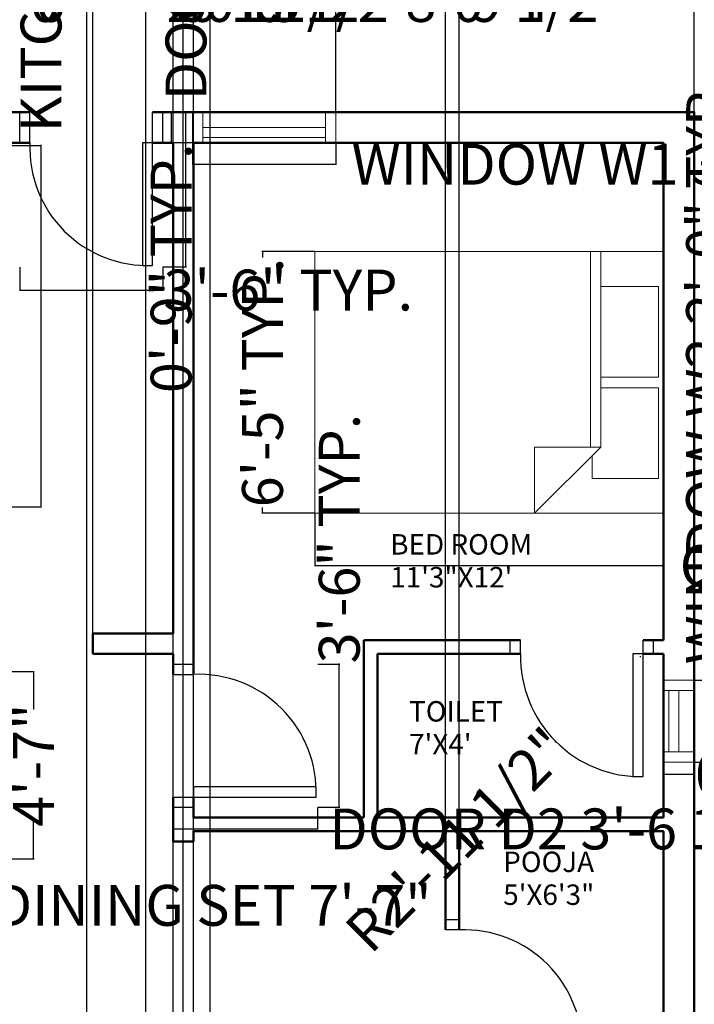
# Model space of a CAD drawing. Units: inches. Extents: x -51 to 1118, y -44 to 791.
# Tile 5 of 8: x 142 to 340, y 344 to 633. Entities that reach past the tile are written whole.
import ezdxf

# ---------------------------------------------------------------- set-up
doc = ezdxf.new("R2010")
doc.units = ezdxf.units.IN
doc.header["$MEASUREMENT"] = 0
for name, color, linetype, lineweight in [('A-ANNO-DIMS', 2, 'Continuous', 18), ('A-AREA-IDEN', 7, 'Continuous', 18), ('A-DOOR', 3, 'Continuous', 25), ('A-FURN', 8, 'Continuous', 18), ('A-GLAZ', 4, 'Continuous', 18), ('A-WALL', 7, 'Continuous', 50)]:
    doc.layers.add(name, color=color, linetype=linetype, lineweight=lineweight)
doc.styles.get("Standard").update_dxf_attribs({"font": 'arial.ttf'})
doc.dimstyles.get("Standard").update_dxf_attribs({"dimtxt": 12, "dimasz": 0.18, "dimexe": 0.18, "dimexo": 0.0625, "dimgap": 0.09, "dimtad": 0, "dimdec": 1, "dimzin": 0, "dimdsep": 46, "dimlunit": 3, "dimtxsty": 'Standard', "dimcen": 0.09, "dimadec": 0, "dimazin": 0, "dimtfac": 1, "dimtdec": 1, "dimtofl": 0, "dimtmove": 0, "dimatfit": 3, "dimfxl": 1, "dimtolj": 1, "dimtzin": 0, "dimarcsym": 0})

# ---------------------------------------------------------------- blocks, each defined once
blk = doc.blocks.new('Bed - Queen')
for p, q in [((0, -80.00003), (0, 0)), ((0, 0), (59.99999, 0)), ((59.99999, 0), (59.99999, -80.00003)), ((7.99999, -1.2), (28.79998, -1.2)), ((7.99999, -14.4), (7.99999, -1.2)), ((28.79998, -1.2), (28.79998, -14.4)), ((31.19999, -1.2), (51.99999, -1.2)), ((31.19999, -14.4), (31.19999, -1.2)), ((51.99999, -1.2), (51.99999, -16.4)), ((0, -14.4), (44.8, -14.4)), ((59.99999, -29.6), (44.8, -14.4)), ((44.8, -14.4), (44.8, -29.6)), ((44.8, -16.8), (0, -16.8)), ((51.99999, -16.4), (46.79936, -16.4)), ((44.8, -29.6), (59.99999, -29.6)), ((59.99999, -80.00003), (0, -80.00003))]:
    blk.add_line(p, q)
blk = doc.blocks.new('*D10')
at = {"layer": 'A-ANNO-DIMS', "color": 0, "lineweight": -2, "transparency": 16777216}
for p, q in [((28.02, 606), (28.02, 654.38)), ((28.2, 654.2), (173.65, 654.2)), ((339.84, 654.2), (194.4, 654.2)), ((340.02, 606), (340.02, 654.38))]:
    blk.add_line(p, q, dxfattribs=at)
at = {"layer": 'A-ANNO-DIMS', "color": 0, "transparency": 16777216}
for points in [[(28.2, 654.23), (28.2, 654.17), (28.02, 654.2)], [(339.84, 654.23), (339.84, 654.17), (340.02, 654.2)]]:
    blk.add_solid(points, dxfattribs=at)
at = {"layer": 'Defpoints', "color": 0, "transparency": 16777216}
for p in [(340.02, 654.2), (28.02, 605.94), (340.02, 605.94)]:
    blk.add_point(p, dxfattribs=at)
at = {"layer": 'A-ANNO-DIMS', "color": 0, "transparency": 16777216, "insert": (184.02, 654.2), "char_height": 12, "attachment_point": 5}
blk.add_mtext("\\A1;26'", dxfattribs=at)
blk = doc.blocks.new('WIN-36IN')
for p, q in [((9, 42), (0, 42)), ((9, 39), (0, 39)), ((0, 39), (0, 3)), ((4.5, 3), (4.5, 39)), ((7.5, 3), (7.5, 39)), ((9, 3), (9, 39)), ((0, 3), (9, 3)), ((0, 0), (9, 0))]:
    blk.add_line(p, q)
blk = doc.blocks.new('WIN-18IN')
for p, q in [((9, 24), (0, 24)), ((0, 21), (0, 3)), ((9, 21), (0, 21)), ((1.5, 21), (1.5, 3)), ((4.5, 21), (4.5, 3)), ((9, 3), (9, 21)), ((0, 3), (9, 3)), ((0, 0), (9, 0))]:
    blk.add_line(p, q)
blk = doc.blocks.new('DOOR-36IN-FRAME-9IN')
for p, q in [((0, 36.03), (0, 45.03)), ((3, 36.03), (3, 45.03)), ((39, 36.03), (39, 45.03)), ((42, 36.03), (42, 45.03))]:
    blk.add_line(p, q)
blk.add_lwpolyline([(39, 36.03), (36, 36.03), (36, 0.03), (39, 0.03)], close=True)
blk.add_arc((37.5, 34.53), 34.53, 177.5104, 272.4896)
blk = doc.blocks.new('DOOR-36IN-FRAME-6IN')
for p, q in [((0, 42), (6, 42)), ((0, 39), (6, 39)), ((0, 3), (6, 3)), ((0, 0), (6, 0))]:
    blk.add_line(p, q)
blk.add_lwpolyline([(6, 3), (42, 3), (42, 6), (6, 6)], close=True)
blk.add_arc((7.5, 4.5), 34.53, 357.5104, 92.4896)
blk = doc.blocks.new('DOOR-36IN-FRAME-4IN')
for p, q in [((4, 42), (0, 42)), ((4, 39), (0, 39)), ((4, 3), (0, 3)), ((4, 0), (0, 0))]:
    blk.add_line(p, q)
blk.add_lwpolyline([(4, 3), (40, 3), (40, 6), (4, 6)], close=True)
blk.add_arc((5.5, 4.5), 34.53, 357.5104, 92.4896)
blk = doc.blocks.new('*D16')
at = {"layer": 'A-ANNO-DIMS', "color": 0, "lineweight": -2, "transparency": 16777216}
for p, q in [((192.77, 596.88), (192.77, 590.46)), ((234.77, 596.88), (234.77, 590.46)), ((192.95, 590.64), (234.59, 590.64)), ((234.77, 590.64), (234.95, 590.64))]:
    blk.add_line(p, q, dxfattribs=at)
at = {"layer": 'A-ANNO-DIMS', "color": 0, "transparency": 16777216}
for points in [[(192.95, 590.67), (192.95, 590.61), (192.77, 590.64)], [(234.59, 590.67), (234.59, 590.61), (234.77, 590.64)]]:
    blk.add_solid(points, dxfattribs=at)
at = {"layer": 'Defpoints', "color": 0, "transparency": 16777216}
for p in [(192.77, 596.94), (234.77, 596.94), (234.77, 590.64)]:
    blk.add_point(p, dxfattribs=at)
at = {"layer": 'A-ANNO-DIMS', "color": 0, "transparency": 16777216, "insert": (325.87, 590.64), "char_height": 12, "attachment_point": 5}
blk.add_mtext('\\A1;WINDOW W1 3\'-6" TYP.', dxfattribs=at)
blk = doc.blocks.new('*D17')
at = {"layer": 'A-ANNO-DIMS', "color": 0, "lineweight": -2, "transparency": 16777216}
for p, q in [((192.71, 605.94), (186.29, 605.94)), ((186.47, 605.76), (186.47, 597.12)), ((192.71, 596.94), (186.29, 596.94)), ((186.47, 596.94), (186.47, 596.76))]:
    blk.add_line(p, q, dxfattribs=at)
at = {"layer": 'A-ANNO-DIMS', "color": 0, "transparency": 16777216}
for points in [[(186.44, 605.76), (186.5, 605.76), (186.47, 605.94)], [(186.44, 597.12), (186.5, 597.12), (186.47, 596.94)]]:
    blk.add_solid(points, dxfattribs=at)
at = {"layer": 'Defpoints', "color": 0, "transparency": 16777216}
for p in [(192.77, 605.94), (186.47, 596.94), (192.77, 596.94)]:
    blk.add_point(p, dxfattribs=at)
at = {"layer": 'A-ANNO-DIMS', "color": 0, "transparency": 16777216, "insert": (186.47, 560.1), "char_height": 12, "attachment_point": 5, "rotation": 90}
blk.add_mtext('\\A1;0\'-9" TYP.', dxfattribs=at)
blk = doc.blocks.new('*D18')
at = {"layer": 'A-ANNO-DIMS', "color": 0, "lineweight": -2, "transparency": 16777216}
for p, q in [((340.08, 439.22), (343.8, 439.22)), ((343.62, 439.22), (343.62, 439.4)), ((343.62, 415.4), (343.62, 439.04)), ((340.08, 415.22), (343.8, 415.22))]:
    blk.add_line(p, q, dxfattribs=at)
at = {"layer": 'A-ANNO-DIMS', "color": 0, "transparency": 16777216}
for points in [[(343.59, 439.04), (343.65, 439.04), (343.62, 439.22)], [(343.59, 415.4), (343.65, 415.4), (343.62, 415.22)]]:
    blk.add_solid(points, dxfattribs=at)
at = {"layer": 'Defpoints', "color": 0, "transparency": 16777216}
for p in [(340.02, 439.22), (343.62, 439.22), (340.02, 415.22)]:
    blk.add_point(p, dxfattribs=at)
at = {"layer": 'A-ANNO-DIMS', "color": 0, "transparency": 16777216, "insert": (343.62, 530.31), "char_height": 12, "attachment_point": 5, "rotation": 90}
blk.add_mtext('\\A1;WINDOW W2 2\'-0" TYP.', dxfattribs=at)
blk = doc.blocks.new('*D19')
at = {"layer": 'A-ANNO-DIMS', "color": 0, "lineweight": -2, "transparency": 16777216}
for p, q in [((331.02, 415.15), (331.02, 411.44)), ((340.02, 415.15), (340.02, 411.44)), ((331.2, 411.62), (339.84, 411.62)), ((340.02, 411.62), (340.2, 411.62))]:
    blk.add_line(p, q, dxfattribs=at)
at = {"layer": 'A-ANNO-DIMS', "color": 0, "transparency": 16777216}
for points in [[(331.2, 411.65), (331.2, 411.59), (331.02, 411.62)], [(339.84, 411.65), (339.84, 411.59), (340.02, 411.62)]]:
    blk.add_solid(points, dxfattribs=at)
at = {"layer": 'Defpoints', "color": 0, "transparency": 16777216}
for p in [(331.02, 415.22), (340.02, 415.22), (340.02, 411.62)]:
    blk.add_point(p, dxfattribs=at)
at = {"layer": 'A-ANNO-DIMS', "color": 0, "transparency": 16777216, "insert": (376.86, 411.62), "char_height": 12, "attachment_point": 5}
blk.add_mtext('\\A1;0\'-9" TYP.', dxfattribs=at)
blk = doc.blocks.new('*D20')
at = {"layer": 'A-ANNO-DIMS', "color": 0, "lineweight": -2, "transparency": 16777216}
for p, q in [((184.08, 605.94), (191.01, 605.94)), ((190.83, 605.94), (190.83, 606.12)), ((190.83, 560.7), (190.83, 605.76)), ((184.08, 560.52), (191.01, 560.52))]:
    blk.add_line(p, q, dxfattribs=at)
at = {"layer": 'A-ANNO-DIMS', "color": 0, "transparency": 16777216}
for points in [[(190.8, 605.76), (190.86, 605.76), (190.83, 605.94)], [(190.8, 560.7), (190.86, 560.7), (190.83, 560.52)]]:
    blk.add_solid(points, dxfattribs=at)
at = {"layer": 'Defpoints', "color": 0, "transparency": 16777216}
for p in [(184.02, 605.94), (190.83, 605.94), (184.02, 560.52)]:
    blk.add_point(p, dxfattribs=at)
at = {"layer": 'A-ANNO-DIMS', "color": 0, "transparency": 16777216, "insert": (190.83, 696.98), "char_height": 12, "attachment_point": 5, "rotation": 90}
blk.add_mtext('\\A1;DOOR D1 3\'-9 1/2" TYP.', dxfattribs=at)
blk = doc.blocks.new('*D21')
at = {"layer": 'A-ANNO-DIMS', "color": 0, "lineweight": -2, "transparency": 16777216}
for p, q in [((142.02, 560.46), (142.02, 553.53)), ((184.02, 560.46), (184.02, 553.53)), ((142.2, 553.71), (183.84, 553.71)), ((184.02, 553.71), (184.2, 553.71))]:
    blk.add_line(p, q, dxfattribs=at)
at = {"layer": 'A-ANNO-DIMS', "color": 0, "transparency": 16777216}
for points in [[(142.2, 553.74), (142.2, 553.68), (142.02, 553.71)], [(183.84, 553.74), (183.84, 553.68), (184.02, 553.71)]]:
    blk.add_solid(points, dxfattribs=at)
at = {"layer": 'Defpoints', "color": 0, "transparency": 16777216}
for p in [(142.02, 560.52), (184.02, 560.52), (184.02, 553.71)]:
    blk.add_point(p, dxfattribs=at)
at = {"layer": 'A-ANNO-DIMS', "color": 0, "transparency": 16777216, "insert": (220.86, 553.71), "char_height": 12, "attachment_point": 5}
blk.add_mtext('\\A1;3\'-6" TYP.', dxfattribs=at)
blk = doc.blocks.new('*D22')
at = {"layer": 'A-ANNO-DIMS', "color": 0, "lineweight": -2, "transparency": 16777216}
for p, q in [((187.02, 401.88), (187.02, 395.4)), ((229.44, 401.88), (229.44, 395.4)), ((187.2, 395.58), (229.26, 395.58)), ((229.44, 395.58), (229.62, 395.58))]:
    blk.add_line(p, q, dxfattribs=at)
at = {"layer": 'A-ANNO-DIMS', "color": 0, "transparency": 16777216}
for points in [[(187.2, 395.61), (187.2, 395.55), (187.02, 395.58)], [(229.26, 395.61), (229.26, 395.55), (229.44, 395.58)]]:
    blk.add_solid(points, dxfattribs=at)
at = {"layer": 'Defpoints', "color": 0, "transparency": 16777216}
for p in [(187.02, 401.94), (229.44, 401.94), (229.44, 395.58)]:
    blk.add_point(p, dxfattribs=at)
at = {"layer": 'A-ANNO-DIMS', "color": 0, "transparency": 16777216, "insert": (320.49, 395.58), "char_height": 12, "attachment_point": 5}
blk.add_mtext('\\A1;DOOR D2 3\'-6 1/2" TYP.', dxfattribs=at)
blk = doc.blocks.new('*D23')
at = {"layer": 'A-ANNO-DIMS', "color": 0, "lineweight": -2, "transparency": 16777216}
for p, q in [((229.5, 443.94), (235.99, 443.94)), ((235.81, 443.94), (235.81, 444.12)), ((235.81, 402.12), (235.81, 443.76)), ((229.5, 401.94), (235.99, 401.94))]:
    blk.add_line(p, q, dxfattribs=at)
at = {"layer": 'A-ANNO-DIMS', "color": 0, "transparency": 16777216}
for points in [[(235.78, 443.76), (235.84, 443.76), (235.81, 443.94)], [(235.78, 402.12), (235.84, 402.12), (235.81, 401.94)]]:
    blk.add_solid(points, dxfattribs=at)
at = {"layer": 'Defpoints', "color": 0, "transparency": 16777216}
for p in [(229.44, 443.94), (235.81, 443.94), (229.44, 401.94)]:
    blk.add_point(p, dxfattribs=at)
at = {"layer": 'A-ANNO-DIMS', "color": 0, "transparency": 16777216, "insert": (235.81, 480.78), "char_height": 12, "attachment_point": 5, "rotation": 90}
blk.add_mtext('\\A1;3\'-6" TYP.', dxfattribs=at)
blk = doc.blocks.new('*D26')
at = {"layer": 'A-ANNO-DIMS', "color": 0, "lineweight": -2, "transparency": 16777216}
for p, q in [((228.63, 488.13), (228.63, 472.66)), ((331.02, 488.13), (331.02, 472.66)), ((228.81, 472.84), (330.84, 472.84)), ((331.02, 472.84), (331.2, 472.84))]:
    blk.add_line(p, q, dxfattribs=at)
at = {"layer": 'A-ANNO-DIMS', "color": 0, "transparency": 16777216}
for points in [[(228.81, 472.87), (228.81, 472.81), (228.63, 472.84)], [(330.84, 472.87), (330.84, 472.81), (331.02, 472.84)]]:
    blk.add_solid(points, dxfattribs=at)
at = {"layer": 'Defpoints', "color": 0, "transparency": 16777216}
for p in [(228.63, 488.2), (331.02, 488.2), (331.02, 472.84)]:
    blk.add_point(p, dxfattribs=at)
at = {"layer": 'A-ANNO-DIMS', "color": 0, "transparency": 16777216, "insert": (433.53, 472.84), "char_height": 12, "attachment_point": 5}
blk.add_mtext('\\A1;QUEEN BED 8\'-6 1/2" TYP.', dxfattribs=at)
blk = doc.blocks.new('*D27')
at = {"layer": 'A-ANNO-DIMS', "color": 0, "lineweight": -2, "transparency": 16777216}
for p, q in [((228.57, 564.99), (213.09, 564.99)), ((213.27, 564.81), (213.27, 563.29)), ((213.27, 488.38), (213.27, 489.9)), ((228.57, 488.2), (213.09, 488.2))]:
    blk.add_line(p, q, dxfattribs=at)
at = {"layer": 'A-ANNO-DIMS', "color": 0, "transparency": 16777216}
for points in [[(213.24, 564.81), (213.3, 564.81), (213.27, 564.99)], [(213.24, 488.38), (213.3, 488.38), (213.27, 488.2)]]:
    blk.add_solid(points, dxfattribs=at)
at = {"layer": 'Defpoints', "color": 0, "transparency": 16777216}
for p in [(228.63, 564.99), (213.27, 488.2), (228.63, 488.2)]:
    blk.add_point(p, dxfattribs=at)
at = {"layer": 'A-ANNO-DIMS', "color": 0, "transparency": 16777216, "insert": (213.27, 526.59), "char_height": 12, "attachment_point": 5, "rotation": 90}
blk.add_mtext('\\A1;6\'-5" TYP.', dxfattribs=at)
blk = doc.blocks.new('*D34')
at = {"layer": 'A-ANNO-DIMS', "color": 0, "lineweight": -2, "transparency": 16777216}
for p, q in [((132.45, 596.14), (148.46, 596.14)), ((148.28, 596.14), (148.28, 596.32)), ((148.28, 490.32), (148.28, 595.96)), ((132.45, 490.14), (148.46, 490.14))]:
    blk.add_line(p, q, dxfattribs=at)
at = {"layer": 'A-ANNO-DIMS', "color": 0, "transparency": 16777216}
for points in [[(148.25, 595.96), (148.31, 595.96), (148.28, 596.14)], [(148.25, 490.32), (148.31, 490.32), (148.28, 490.14)]]:
    blk.add_solid(points, dxfattribs=at)
at = {"layer": 'Defpoints', "color": 0, "transparency": 16777216}
for p in [(132.38, 596.14), (148.28, 596.14), (132.38, 490.14)]:
    blk.add_point(p, dxfattribs=at)
at = {"layer": 'A-ANNO-DIMS', "color": 0, "transparency": 16777216, "insert": (148.28, 696.39), "char_height": 12, "attachment_point": 5, "rotation": 90}
blk.add_mtext('\\A1;KITCHEN FITTINGS 8\'-10"', dxfattribs=at)
blk = doc.blocks.new('*D40')
at = {"layer": 'A-ANNO-DIMS', "color": 0, "lineweight": -2, "transparency": 16777216}
for p, q in [((41.43, 386.75), (41.43, 372.98)), ((132.43, 386.75), (132.43, 372.98)), ((41.61, 373.16), (132.25, 373.16)), ((132.43, 373.16), (132.61, 373.16))]:
    blk.add_line(p, q, dxfattribs=at)
at = {"layer": 'A-ANNO-DIMS', "color": 0, "transparency": 16777216}
for points in [[(41.61, 373.19), (41.61, 373.13), (41.43, 373.16)], [(132.25, 373.19), (132.25, 373.13), (132.43, 373.16)]]:
    blk.add_solid(points, dxfattribs=at)
at = {"layer": 'Defpoints', "color": 0, "transparency": 16777216}
for p in [(41.43, 386.81), (132.43, 386.81), (132.43, 373.16)]:
    blk.add_point(p, dxfattribs=at)
at = {"layer": 'A-ANNO-DIMS', "color": 0, "transparency": 16777216, "insert": (198.65, 373.16), "char_height": 12, "attachment_point": 5}
blk.add_mtext('\\A1;DINING SET 7\'-7"', dxfattribs=at)
blk = doc.blocks.new('*D41')
at = {"layer": 'A-ANNO-DIMS', "color": 0, "lineweight": -2, "transparency": 16777216}
for p, q in [((132.49, 441.81), (146.26, 441.81)), ((146.08, 441.63), (146.08, 430.59)), ((146.08, 386.99), (146.08, 398.03)), ((132.49, 386.81), (146.26, 386.81))]:
    blk.add_line(p, q, dxfattribs=at)
at = {"layer": 'A-ANNO-DIMS', "color": 0, "transparency": 16777216}
for points in [[(146.05, 441.63), (146.11, 441.63), (146.08, 441.81)], [(146.05, 386.99), (146.11, 386.99), (146.08, 386.81)]]:
    blk.add_solid(points, dxfattribs=at)
at = {"layer": 'Defpoints', "color": 0, "transparency": 16777216}
for p in [(132.43, 441.81), (146.08, 441.81), (132.43, 386.81)]:
    blk.add_point(p, dxfattribs=at)
at = {"layer": 'A-ANNO-DIMS', "color": 0, "transparency": 16777216, "insert": (146.08, 414.31), "char_height": 12, "attachment_point": 5, "rotation": 90}
blk.add_mtext('\\A1;4\'-7"', dxfattribs=at)
blk = doc.blocks.new('*D43')
at = {"layer": 'A-ANNO-DIMS', "color": 0, "lineweight": -2, "transparency": 16777216}
for p, q in [((187.02, 597), (187.02, 638.57)), ((193.02, 597), (193.02, 638.57)), ((187.2, 638.39), (192.84, 638.39)), ((193.02, 638.39), (193.2, 638.39))]:
    blk.add_line(p, q, dxfattribs=at)
at = {"layer": 'A-ANNO-DIMS', "color": 0, "transparency": 16777216}
for points in [[(187.2, 638.42), (187.2, 638.36), (187.02, 638.39)], [(192.84, 638.42), (192.84, 638.36), (193.02, 638.39)]]:
    blk.add_solid(points, dxfattribs=at)
at = {"layer": 'Defpoints', "color": 0, "transparency": 16777216}
for p in [(193.02, 638.39), (187.02, 596.94), (193.02, 596.94)]:
    blk.add_point(p, dxfattribs=at)
at = {"layer": 'A-ANNO-DIMS', "color": 0, "transparency": 16777216, "insert": (209.24, 638.39), "char_height": 12, "attachment_point": 5}
blk.add_mtext('\\A1;0\'-6"', dxfattribs=at)
blk = doc.blocks.new('*D49')
at = {"layer": 'A-ANNO-DIMS', "color": 0, "lineweight": -2, "transparency": 16777216}
for p, q in [((234.77, 606), (234.77, 638.57)), ((340.02, 606), (340.02, 638.57)), ((234.95, 638.39), (257.37, 638.39)), ((339.84, 638.39), (317.42, 638.39))]:
    blk.add_line(p, q, dxfattribs=at)
at = {"layer": 'A-ANNO-DIMS', "color": 0, "transparency": 16777216}
for points in [[(234.95, 638.42), (234.95, 638.36), (234.77, 638.39)], [(339.84, 638.42), (339.84, 638.36), (340.02, 638.39)]]:
    blk.add_solid(points, dxfattribs=at)
at = {"layer": 'Defpoints', "color": 0, "transparency": 16777216}
for p in [(340.02, 638.39), (234.77, 605.94), (340.02, 605.94)]:
    blk.add_point(p, dxfattribs=at)
at = {"layer": 'A-ANNO-DIMS', "color": 0, "transparency": 16777216, "insert": (287.4, 638.39), "char_height": 12, "attachment_point": 5}
blk.add_mtext('\\A1;8\'-9 1/2"', dxfattribs=at)
blk = doc.blocks.new('*D52')
at = {"layer": 'A-ANNO-DIMS', "color": 0, "lineweight": -2, "transparency": 16777216}
for p, q in [((340.08, 415.22), (372.65, 415.22)), ((372.47, 415.04), (372.47, 375.54)), ((372.47, 267.81), (372.47, 307.31)), ((340.08, 267.63), (372.65, 267.63))]:
    blk.add_line(p, q, dxfattribs=at)
at = {"layer": 'A-ANNO-DIMS', "color": 0, "transparency": 16777216}
for points in [[(372.44, 415.04), (372.5, 415.04), (372.47, 415.22)], [(372.44, 267.81), (372.5, 267.81), (372.47, 267.63)]]:
    blk.add_solid(points, dxfattribs=at)
at = {"layer": 'Defpoints', "color": 0, "transparency": 16777216}
for p in [(340.02, 415.22), (372.47, 415.22), (340.02, 267.63)]:
    blk.add_point(p, dxfattribs=at)
at = {"layer": 'A-ANNO-DIMS', "color": 0, "transparency": 16777216, "insert": (372.47, 341.42), "char_height": 12, "attachment_point": 5, "rotation": 90}
blk.add_mtext('\\A1;12\'-3 1/2"', dxfattribs=at)
blk = doc.blocks.new('*D55')
at = {"layer": 'A-ANNO-DIMS', "color": 0, "lineweight": -2, "transparency": 16777216}
for p, q in [((193.02, 108), (193.02, 638.57)), ((197.97, 108), (197.97, 638.57)), ((193.2, 638.39), (197.79, 638.39)), ((197.97, 638.39), (198.15, 638.39))]:
    blk.add_line(p, q, dxfattribs=at)
at = {"layer": 'A-ANNO-DIMS', "color": 0, "transparency": 16777216}
for points in [[(193.2, 638.42), (193.2, 638.36), (193.02, 638.39)], [(197.79, 638.42), (197.79, 638.36), (197.97, 638.39)]]:
    blk.add_solid(points, dxfattribs=at)
at = {"layer": 'Defpoints', "color": 0, "transparency": 16777216}
for p in [(197.97, 638.39), (193.02, 107.94), (197.97, 107.94)]:
    blk.add_point(p, dxfattribs=at)
at = {"layer": 'A-ANNO-DIMS', "color": 0, "transparency": 16777216, "insert": (214.19, 638.39), "char_height": 12, "attachment_point": 5}
blk.add_mtext('\\A1;0\'-5"', dxfattribs=at)
blk = doc.blocks.new('*D57')
at = {"layer": 'A-ANNO-DIMS', "color": 0, "lineweight": -2, "transparency": 16777216}
for p, q in [((179.02, 57), (179.02, 638.57)), ((190.02, 57), (190.02, 638.57)), ((179.2, 638.39), (189.84, 638.39)), ((190.02, 638.39), (190.2, 638.39))]:
    blk.add_line(p, q, dxfattribs=at)
at = {"layer": 'A-ANNO-DIMS', "color": 0, "transparency": 16777216}
for points in [[(179.2, 638.42), (179.2, 638.36), (179.02, 638.39)], [(189.84, 638.42), (189.84, 638.36), (190.02, 638.39)]]:
    blk.add_solid(points, dxfattribs=at)
at = {"layer": 'Defpoints', "color": 0, "transparency": 16777216}
for p in [(190.02, 638.39), (179.02, 56.94), (190.02, 56.94)]:
    blk.add_point(p, dxfattribs=at)
at = {"layer": 'A-ANNO-DIMS', "color": 0, "transparency": 16777216, "insert": (210.9, 638.39), "char_height": 12, "attachment_point": 5}
blk.add_mtext('\\A1;0\'-11"', dxfattribs=at)
blk = doc.blocks.new('*D61')
at = {"layer": 'A-ANNO-DIMS', "color": 0, "lineweight": -2, "transparency": 16777216}
for p, q in [((125.75, 324), (125.75, 638.57)), ((161.75, 324), (161.75, 638.57)), ((125.93, 638.39), (127.71, 638.39)), ((161.57, 638.39), (159.79, 638.39))]:
    blk.add_line(p, q, dxfattribs=at)
at = {"layer": 'A-ANNO-DIMS', "color": 0, "transparency": 16777216}
for points in [[(125.93, 638.42), (125.93, 638.36), (125.75, 638.39)], [(161.57, 638.42), (161.57, 638.36), (161.75, 638.39)]]:
    blk.add_solid(points, dxfattribs=at)
at = {"layer": 'Defpoints', "color": 0, "transparency": 16777216}
for p in [(161.75, 638.39), (125.75, 323.94), (161.75, 323.94)]:
    blk.add_point(p, dxfattribs=at)
at = {"layer": 'A-ANNO-DIMS', "color": 0, "transparency": 16777216, "insert": (143.75, 638.39), "char_height": 12, "attachment_point": 5}
blk.add_mtext('\\A1;3\'-0"', dxfattribs=at)
blk = doc.blocks.new('*D62')
at = {"layer": 'A-ANNO-DIMS', "color": 0, "lineweight": -2, "transparency": 16777216}
for p, q in [((161.75, 324), (161.75, 638.57)), ((187.02, 327), (187.02, 638.57)), ((161.93, 638.39), (186.84, 638.39)), ((187.02, 638.39), (187.2, 638.39))]:
    blk.add_line(p, q, dxfattribs=at)
at = {"layer": 'A-ANNO-DIMS', "color": 0, "transparency": 16777216}
for points in [[(161.93, 638.42), (161.93, 638.36), (161.75, 638.39)], [(186.84, 638.42), (186.84, 638.36), (187.02, 638.39)]]:
    blk.add_solid(points, dxfattribs=at)
at = {"layer": 'Defpoints', "color": 0, "transparency": 16777216}
for p in [(187.02, 638.39), (187.02, 326.94), (161.75, 323.94)]:
    blk.add_point(p, dxfattribs=at)
at = {"layer": 'A-ANNO-DIMS', "color": 0, "transparency": 16777216, "insert": (217.32, 638.39), "char_height": 12, "attachment_point": 5}
blk.add_mtext('\\A1;2\'-1 1/2"', dxfattribs=at)
blk = doc.blocks.new('*D63')
at = {"layer": 'A-ANNO-DIMS', "color": 0, "lineweight": -2, "transparency": 16777216}
for p, q in [((127.45, 453), (127.45, 638.57)), ((163.45, 453), (163.45, 638.57)), ((127.63, 638.39), (129.41, 638.39)), ((163.27, 638.39), (161.48, 638.39))]:
    blk.add_line(p, q, dxfattribs=at)
at = {"layer": 'A-ANNO-DIMS', "color": 0, "transparency": 16777216}
for points in [[(127.63, 638.42), (127.63, 638.36), (127.45, 638.39)], [(163.27, 638.42), (163.27, 638.36), (163.45, 638.39)]]:
    blk.add_solid(points, dxfattribs=at)
at = {"layer": 'Defpoints', "color": 0, "transparency": 16777216}
for p in [(163.45, 638.39), (127.45, 452.94), (163.45, 452.94)]:
    blk.add_point(p, dxfattribs=at)
at = {"layer": 'A-ANNO-DIMS', "color": 0, "transparency": 16777216, "insert": (145.45, 638.39), "char_height": 12, "attachment_point": 5}
blk.add_mtext('\\A1;3\'-0"', dxfattribs=at)
blk = doc.blocks.new('*D64')
at = {"layer": 'A-ANNO-DIMS', "color": 0, "lineweight": -2, "transparency": 16777216}
for p, q in [((163.45, 453), (163.45, 638.57)), ((187.02, 453), (187.02, 638.57)), ((163.63, 638.39), (186.84, 638.39)), ((187.02, 638.39), (187.2, 638.39))]:
    blk.add_line(p, q, dxfattribs=at)
at = {"layer": 'A-ANNO-DIMS', "color": 0, "transparency": 16777216}
for points in [[(163.63, 638.42), (163.63, 638.36), (163.45, 638.39)], [(186.84, 638.42), (186.84, 638.36), (187.02, 638.39)]]:
    blk.add_solid(points, dxfattribs=at)
at = {"layer": 'Defpoints', "color": 0, "transparency": 16777216}
for p in [(187.02, 638.39), (163.45, 452.94), (187.02, 452.94)]:
    blk.add_point(p, dxfattribs=at)
at = {"layer": 'A-ANNO-DIMS', "color": 0, "transparency": 16777216, "insert": (221.32, 638.39), "char_height": 12, "attachment_point": 5}
blk.add_mtext('\\A1;1\'-11 1/2"', dxfattribs=at)
blk = doc.blocks.new('*D65')
at = {"layer": 'A-ANNO-DIMS', "color": 0, "lineweight": -2, "transparency": 16777216}
for p, q in [((267.02, 366), (267.02, 638.57)), ((271.02, 366), (271.02, 638.57)), ((267.2, 638.39), (270.84, 638.39)), ((271.02, 638.39), (271.2, 638.39))]:
    blk.add_line(p, q, dxfattribs=at)
at = {"layer": 'A-ANNO-DIMS', "color": 0, "transparency": 16777216}
for points in [[(267.2, 638.42), (267.2, 638.36), (267.02, 638.39)], [(270.84, 638.42), (270.84, 638.36), (271.02, 638.39)]]:
    blk.add_solid(points, dxfattribs=at)
at = {"layer": 'Defpoints', "color": 0, "transparency": 16777216}
for p in [(271.02, 638.39), (267.02, 365.94), (271.02, 365.94)]:
    blk.add_point(p, dxfattribs=at)
at = {"layer": 'A-ANNO-DIMS', "color": 0, "transparency": 16777216, "insert": (287.24, 638.39), "char_height": 12, "attachment_point": 5}
blk.add_mtext('\\A1;0\'-4"', dxfattribs=at)
blk = doc.blocks.new('*D66')
at = {"layer": 'A-ANNO-DIMS', "color": 0, "lineweight": -2, "transparency": 16777216}
for p, q in [((324.18, 446.19), (324.36, 446.19)), ((324.27, 446.1), (324.27, 446.28)), ((299.09, 421), (299.21, 421.13))]:
    blk.add_line(p, q, dxfattribs=at)
at = {"layer": 'A-ANNO-DIMS', "color": 0, "transparency": 16777216}
blk.add_solid([(299.19, 421.15), (299.23, 421.11), (299.34, 421.26)], dxfattribs=at)
at = {"layer": 'Defpoints', "color": 0, "transparency": 16777216}
for p in [(324.27, 446.19), (299.34, 421.26)]:
    blk.add_point(p, dxfattribs=at)
at = {"layer": 'A-ANNO-DIMS', "color": 0, "transparency": 16777216, "insert": (270.5, 392.42), "char_height": 12, "attachment_point": 5, "rotation": 45.0007}
blk.add_mtext('\\A1;R2\'-11 1/2"', dxfattribs=at)

msp = doc.modelspace()

# ---------------------------------------------------------------- linework, layer by layer
at = {"layer": 'A-DOOR'}
for p, q in [((286.02, 446.94), (286.02, 450.94)), ((289.02, 446.94), (289.02, 450.94)), ((325.02, 446.94), (325.02, 450.94)), ((328.02, 446.94), (328.02, 450.94))]:
    msp.add_line(p, q, dxfattribs=at)
msp.add_lwpolyline([(325.02, 446.94), (322.02, 446.94), (322.02, 410.94), (325.02, 410.94)], close=True, dxfattribs=at)
msp.add_arc((324.27, 446.19), 35.26, 178.7811, 271.2189, dxfattribs=at)
at = {"layer": 'A-WALL'}
for p, q in [((145.02, 596.94), (37.02, 596.94)), ((187.02, 596.94), (181.02, 596.94)), ((187.02, 596.94), (187.02, 452.94)), ((331.02, 596.94), (193.02, 596.94)), ((193.02, 596.94), (193.02, 440.94)), ((331.02, 450.94), (331.02, 596.94)), ((187.02, 452.94), (163.45, 452.94)), ((163.45, 446.94), (163.45, 452.94)), ((243.02, 398.94), (243.02, 450.94)), ((289.02, 450.94), (243.02, 450.94)), ((331.02, 450.94), (325.02, 450.94)), ((187.02, 446.94), (163.45, 446.94)), ((187.02, 446.94), (187.02, 440.94)), ((193.02, 446.94), (193.02, 440.94)), ((247.02, 398.94), (247.02, 446.94)), ((289.02, 446.94), (247.02, 446.94)), ((331.02, 446.94), (325.02, 446.94)), ((331.02, 398.94), (331.02, 446.94)), ((187.02, 391.94), (187.02, 404.94)), ((193.02, 404.94), (193.02, 398.94)), ((193.02, 404.94), (193.02, 398.94)), ((243.02, 398.94), (193.02, 398.94)), ((331.02, 398.94), (247.02, 398.94)), ((331.02, 394.94), (193.02, 394.94)), ((193.02, 391.94), (193.02, 394.94)), ((267.02, 365.94), (267.02, 394.94)), ((271.02, 365.94), (271.02, 394.94)), ((331.02, 323.94), (331.02, 394.94)), ((193.02, 391.94), (187.02, 391.94))]:
    msp.add_line(p, q, dxfattribs=at)
msp.add_lwpolyline([(145.02, 605.94), (28.02, 605.94), (28.02, 5.94), (340.02, 5.94), (340.02, 605.94), (181.02, 605.94)], dxfattribs=at)

# ---------------------------------------------------------------- block references
at = {"layer": 'A-DOOR'}
for name, p in [('DOOR-36IN-FRAME-9IN', (142.02, 560.91)), ('DOOR-36IN-FRAME-6IN', (187.02, 401.94)), ('DOOR-36IN-FRAME-4IN', (267.02, 326.94))]:
    msp.add_blockref(name, p, dxfattribs=at)
at = {"layer": 'A-FURN', "xscale": 1.279882060607878, "yscale": 1.279882060607878, "zscale": 1.279882060607878, "rotation": 270}
msp.add_blockref('Bed - Queen', (331.02, 564.99), dxfattribs=at)
at = {"layer": 'A-GLAZ', "rotation": 270.0000000000001}
msp.add_blockref('WIN-36IN', (192.77, 605.94), dxfattribs=at)
at = {"layer": 'A-GLAZ'}
msp.add_blockref('WIN-18IN', (331.02, 415.22), dxfattribs=at)

# ---------------------------------------------------------------- texts
at = {"layer": 'A-AREA-IDEN'}
for s, p in [('BED ROOM', (250.78, 476.09)), ('11\'3"X12\'', (250.78, 466.45)), ('TOILET', (256.31, 427.09)), ("7'X4'", (256.31, 417.46)), ('POOJA', (283.93, 382.93)), ('5\'X6\'3"', (283.93, 373.29))]:
    msp.add_text(s, height=6, dxfattribs=at).set_placement(p)

# ---------------------------------------------------------------- dimensions: what is measured, and where the dimension line sits
at = {"layer": 'A-ANNO-DIMS'}
for base, p1, p2, angle, text, picture, middle in [((148.28, 596.14), (132.38, 490.14), (132.38, 596.14), 90, 'KITCHEN FITTINGS <>', '*D34', (148.28, 696.39)), ((190.83, 605.94), (184.02, 560.52), (184.02, 605.94), 90, 'DOOR D1 <> TYP.', '*D20', (190.83, 696.98)), ((234.77, 590.64), (192.77, 596.94), (234.77, 596.94), 0, 'WINDOW W1 <> TYP.', '*D16', (325.87, 590.64)), ((343.62, 439.22), (340.02, 415.22), (340.02, 439.22), 90, 'WINDOW W2 <> TYP.', '*D18', (343.62, 530.31)), ((186.47, 596.94), (192.77, 605.94), (192.77, 596.94), 270, '<> TYP.', '*D17', (186.47, 560.1)), ((213.27, 488.2), (228.63, 564.99), (228.63, 488.2), 270, '<> TYP.', '*D27', (213.27, 526.59)), ((235.81, 443.94), (229.44, 401.94), (229.44, 443.94), 90, '<> TYP.', '*D23', (235.81, 480.78))]:
    dim = msp.add_linear_dim(base=base, p1=p1, p2=p2, angle=angle, text=text, dimstyle='Standard', override={"dimdec": 1, "dimlfac": 1, "dimrnd": 0, "dimzin": 1, "dimdsep": 46, "dimlunit": 4, "dimfrac": 2}, dxfattribs=at)
    dim.commit()
    dim.dimension.update_dxf_attribs({"geometry": picture, "text_midpoint": middle})
for base, p1, p2, override, picture, middle in [((340.02, 654.2), (28.02, 605.94), (340.02, 605.94), {"dimclrd": 0, "dimclre": 0, "dimclrt": 0}, '*D10', (184.02, 654.2)), ((187.02, 638.39), (161.75, 323.94), (187.02, 326.94), {"dimdec": 1, "dimlfac": 1, "dimrnd": 0, "dimzin": 1, "dimdsep": 46, "dimlunit": 4, "dimfrac": 2}, '*D62', (217.32, 638.39)), ((187.02, 638.39), (163.45, 452.94), (187.02, 452.94), {"dimdec": 1, "dimlfac": 1, "dimrnd": 0, "dimzin": 1, "dimdsep": 46, "dimlunit": 4, "dimfrac": 2}, '*D64', (221.32, 638.39)), ((340.0217, 638.3903), (234.7701, 605.9403), (340.0217, 605.9403), {"dimdec": 1, "dimlfac": 1, "dimrnd": 0, "dimzin": 1, "dimdsep": 46, "dimlunit": 4, "dimfrac": 2}, '*D49', (287.3959, 638.3903)), ((161.75, 638.39), (125.75, 323.94), (161.75, 323.94), {"dimdec": 1, "dimlfac": 1, "dimrnd": 0, "dimzin": 1, "dimdsep": 46, "dimlunit": 4, "dimfrac": 2}, '*D61', (143.75, 638.39)), ((163.45, 638.39), (127.45, 452.94), (163.45, 452.94), {"dimdec": 1, "dimlfac": 1, "dimrnd": 0, "dimzin": 1, "dimdsep": 46, "dimlunit": 4, "dimfrac": 2}, '*D63', (145.45, 638.39)), ((190.02, 638.39), (179.02, 56.94), (190.02, 56.94), {"dimdec": 1, "dimlfac": 1, "dimrnd": 0, "dimzin": 1, "dimdsep": 46, "dimlunit": 4, "dimfrac": 2}, '*D57', (210.9, 638.39)), ((193.02, 638.39), (187.02, 596.94), (193.02, 596.94), {"dimdec": 1, "dimlfac": 1, "dimrnd": 0, "dimzin": 1, "dimdsep": 46, "dimlunit": 4, "dimfrac": 2}, '*D43', (209.24, 638.39)), ((197.9672, 638.3903), (193.0217, 107.9403), (197.9672, 107.9403), {"dimdec": 1, "dimlfac": 1, "dimrnd": 0, "dimzin": 1, "dimdsep": 46, "dimlunit": 4, "dimfrac": 2}, '*D55', (214.1868, 638.3903)), ((271.02, 638.39), (267.02, 365.94), (271.02, 365.94), {"dimdec": 1, "dimlfac": 1, "dimrnd": 0, "dimzin": 1, "dimdsep": 46, "dimlunit": 4, "dimfrac": 2}, '*D65', (287.24, 638.39))]:
    dim = msp.add_linear_dim(base=base, p1=p1, p2=p2, dimstyle='Standard', override=override, dxfattribs=at)
    dim.commit()
    dim.dimension.update_dxf_attribs({"geometry": picture, "text_midpoint": middle})
for base, p1, p2, text, picture, middle in [((184.02, 553.71), (142.02, 560.52), (184.02, 560.52), '<> TYP.', '*D21', (220.86, 553.71)), ((331.02, 472.84), (228.63, 488.2), (331.02, 488.2), 'QUEEN BED <> TYP.', '*D26', (433.53, 472.84)), ((229.44, 395.58), (187.02, 401.94), (229.44, 401.94), 'DOOR D2 <> TYP.', '*D22', (320.49, 395.58)), ((340.02, 411.62), (331.02, 415.22), (340.02, 415.22), '<> TYP.', '*D19', (376.86, 411.62)), ((132.43, 373.16), (41.43, 386.81), (132.43, 386.81), 'DINING SET <>', '*D40', (198.65, 373.16))]:
    dim = msp.add_linear_dim(base=base, p1=p1, p2=p2, text=text, dimstyle='Standard', override={"dimdec": 1, "dimlfac": 1, "dimrnd": 0, "dimzin": 1, "dimdsep": 46, "dimlunit": 4, "dimfrac": 2}, dxfattribs=at)
    dim.commit()
    dim.dimension.update_dxf_attribs({"geometry": picture, "text_midpoint": middle})
dim = msp.add_radius_dim(center=(324.27, 446.19), mpoint=(299.34, 421.26), dimstyle='Standard', override={"dimdec": 1, "dimlfac": 1, "dimrnd": 0, "dimzin": 1, "dimdsep": 46, "dimlunit": 4, "dimfrac": 2}, dxfattribs=at)
dim.commit()
dim.dimension.update_dxf_attribs({"geometry": '*D66', "text_midpoint": (270.5, 392.42)})
for base, p1, p2, picture, middle in [((146.08, 441.81), (132.43, 386.81), (132.43, 441.81), '*D41', (146.08, 414.31)), ((372.47, 415.22), (340.02, 267.63), (340.02, 415.22), '*D52', (372.47, 341.42))]:
    dim = msp.add_linear_dim(base=base, p1=p1, p2=p2, angle=90, dimstyle='Standard', override={"dimdec": 1, "dimlfac": 1, "dimrnd": 0, "dimzin": 1, "dimdsep": 46, "dimlunit": 4, "dimfrac": 2}, dxfattribs=at)
    dim.commit()
    dim.dimension.update_dxf_attribs({"geometry": picture, "text_midpoint": middle})

doc.saveas('drawing.dxf')
